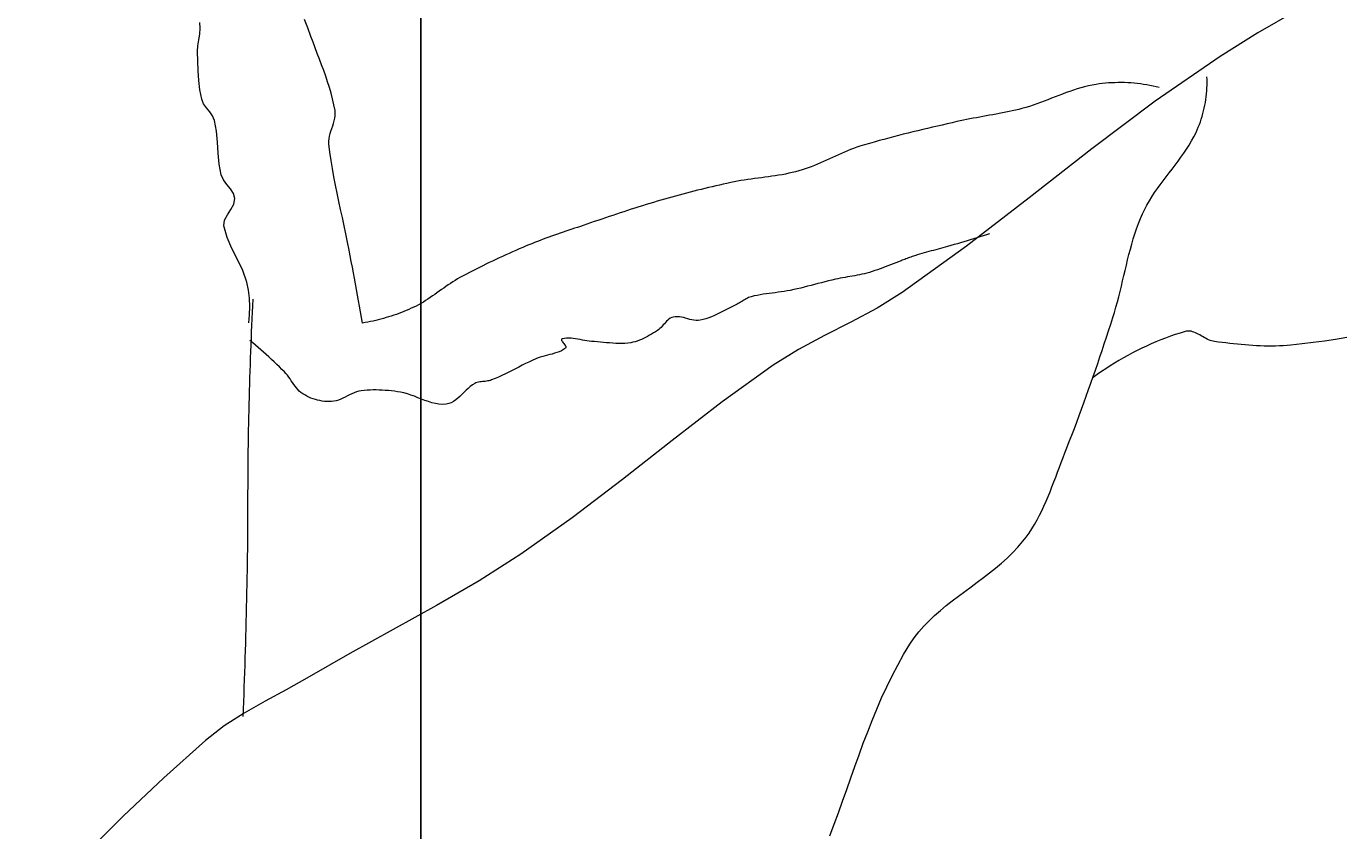
# Model space of a CAD drawing. Units: inches. Extents: x 1770 to 2988, y 1161 to 3221.
# Tile 15 of 44: x 2194 to 2229, y 2323 to 2344. Entities that reach past the tile are written whole.
import ezdxf

# ---------------------------------------------------------------- set-up
doc = ezdxf.new("R2010")
doc.units = ezdxf.units.IN
doc.layers.add('A-ANNO-DIMS', color=2, linetype='Continuous', lineweight=18)
doc.layers.add('A-FURN', color=8, linetype='Continuous', lineweight=13)
doc.styles.get("Standard").update_dxf_attribs({"font": 'arial.ttf'})
doc.dimstyles.get("Standard").update_dxf_attribs({"dimtxt": 0.18, "dimasz": 0.18, "dimexe": 0.18, "dimexo": 0.0625, "dimgap": 0.09, "dimtad": 0, "dimtih": 1, "dimtoh": 1, "dimdec": 4, "dimzin": 0, "dimdsep": 46, "dimtxsty": 'Standard', "dimcen": 0.09, "dimadec": 0, "dimazin": 0, "dimtfac": 1, "dimtdec": 4, "dimtofl": 0, "dimtmove": 0, "dimatfit": 3, "dimfxl": 1, "dimtolj": 1, "dimtzin": 0, "dimarcsym": 0})

# ---------------------------------------------------------------- blocks, each defined once
blk = doc.blocks.new('BED-DOUBLE-PLAN')
for p, q in [((8.372, 84.675), (8.284, 84.904)), ((34.877, 85.131), (33.846, 84.541)), ((5.475, 84.513), (5.49, 84.67)), ((5.49, 84.67), (5.478, 84.825)), ((8.458, 84.444), (8.372, 84.675)), ((33.846, 84.541), (32.841, 83.914)), ((5.415, 84.04), (5.424, 84.198)), ((5.424, 84.198), (5.448, 84.355)), ((5.448, 84.355), (5.475, 84.513)), ((8.513, 84.293), (8.458, 84.444)), ((8.57, 84.142), (8.513, 84.293)), ((5.421, 83.783), (5.415, 84.04)), ((8.628, 83.992), (8.57, 84.142)), ((8.685, 83.841), (8.628, 83.992)), ((8.743, 83.69), (8.685, 83.841)), ((32.841, 83.914), (31.092, 82.71)), ((5.43, 83.526), (5.421, 83.783)), ((5.447, 83.269), (5.43, 83.526)), ((8.799, 83.539), (8.743, 83.69)), ((8.853, 83.387), (8.799, 83.539)), ((5.478, 83.015), (5.447, 83.269)), ((8.905, 83.235), (8.853, 83.387)), ((8.954, 83.082), (8.905, 83.235)), ((29.405, 83.144), (29.303, 83.123)), ((29.508, 83.162), (29.405, 83.144)), ((29.592, 83.174), (29.508, 83.162)), ((29.676, 83.184), (29.592, 83.174)), ((29.761, 83.193), (29.676, 83.184)), ((29.846, 83.2), (29.761, 83.193)), ((29.931, 83.205), (29.846, 83.2)), ((30.016, 83.208), (29.931, 83.205)), ((30.102, 83.21), (30.016, 83.208)), ((30.187, 83.21), (30.102, 83.21)), ((30.273, 83.209), (30.187, 83.21)), ((30.358, 83.205), (30.273, 83.209)), ((30.444, 83.2), (30.358, 83.205)), ((30.529, 83.194), (30.444, 83.2)), ((30.614, 83.185), (30.529, 83.194)), ((30.699, 83.175), (30.614, 83.185)), ((30.784, 83.163), (30.699, 83.175)), ((30.868, 83.15), (30.784, 83.163)), ((30.952, 83.135), (30.868, 83.15)), ((31.036, 83.118), (30.952, 83.135)), ((32.486, 83.292), (32.483, 83.369)), ((32.483, 83.063), (32.486, 83.14)), ((32.487, 83.216), (32.486, 83.292)), ((32.486, 83.14), (32.487, 83.216)), ((5.528, 82.764), (5.478, 83.015)), ((8.999, 82.928), (8.954, 83.082)), ((9.039, 82.773), (8.999, 82.928)), ((9.075, 82.617), (9.039, 82.773)), ((28.314, 82.79), (28.216, 82.752)), ((28.411, 82.829), (28.314, 82.79)), ((28.509, 82.867), (28.411, 82.829)), ((28.607, 82.904), (28.509, 82.867)), ((28.705, 82.941), (28.607, 82.904)), ((28.804, 82.976), (28.705, 82.941)), ((28.902, 83.01), (28.804, 82.976)), ((29.002, 83.042), (28.902, 83.01)), ((29.102, 83.072), (29.002, 83.042)), ((29.202, 83.099), (29.102, 83.072)), ((29.303, 83.123), (29.202, 83.099)), ((31.119, 83.1), (31.036, 83.118)), ((31.201, 83.08), (31.119, 83.1)), ((32.453, 82.757), (32.463, 82.833)), ((32.463, 82.833), (32.472, 82.91)), ((32.472, 82.91), (32.478, 82.986)), ((32.478, 82.986), (32.483, 83.063)), ((5.579, 82.643), (5.528, 82.764)), ((5.656, 82.532), (5.579, 82.643)), ((5.743, 82.426), (5.656, 82.532)), ((5.82, 82.316), (5.743, 82.426)), ((9.104, 82.459), (9.075, 82.617)), ((9.111, 82.39), (9.104, 82.459)), ((27.176, 82.433), (27.089, 82.415)), ((27.263, 82.452), (27.176, 82.433)), ((27.35, 82.472), (27.263, 82.452)), ((27.436, 82.493), (27.35, 82.472)), ((27.522, 82.516), (27.436, 82.493)), ((27.623, 82.544), (27.522, 82.516)), ((27.723, 82.574), (27.623, 82.544)), ((27.822, 82.607), (27.723, 82.574)), ((27.921, 82.642), (27.822, 82.607)), ((28.02, 82.678), (27.921, 82.642)), ((28.118, 82.715), (28.02, 82.678)), ((28.216, 82.752), (28.118, 82.715)), ((31.092, 82.71), (29.393, 81.433)), ((32.374, 82.379), (32.393, 82.454)), ((32.393, 82.454), (32.411, 82.529)), ((32.411, 82.529), (32.427, 82.605)), ((32.427, 82.605), (32.441, 82.68)), ((32.441, 82.68), (32.453, 82.757)), ((5.872, 82.195), (5.82, 82.316)), ((5.926, 81.906), (5.872, 82.195)), ((9.041, 82.049), (9.064, 82.117)), ((9.064, 82.117), (9.083, 82.185)), ((9.083, 82.185), (9.099, 82.253)), ((9.099, 82.253), (9.108, 82.322)), ((9.108, 82.322), (9.111, 82.39)), ((25.385, 82.073), (25.254, 82.042)), ((25.516, 82.103), (25.385, 82.073)), ((25.647, 82.133), (25.516, 82.103)), ((25.778, 82.164), (25.647, 82.133)), ((25.865, 82.183), (25.778, 82.164)), ((25.952, 82.202), (25.865, 82.183)), ((26.039, 82.22), (25.952, 82.202)), ((26.126, 82.237), (26.039, 82.22)), ((26.214, 82.254), (26.126, 82.237)), ((26.301, 82.27), (26.214, 82.254)), ((26.389, 82.286), (26.301, 82.27)), ((26.477, 82.301), (26.389, 82.286)), ((26.564, 82.317), (26.477, 82.301)), ((26.652, 82.333), (26.564, 82.317)), ((26.74, 82.348), (26.652, 82.333)), ((26.827, 82.364), (26.74, 82.348)), ((26.915, 82.381), (26.827, 82.364)), ((27.002, 82.397), (26.915, 82.381)), ((27.089, 82.415), (27.002, 82.397)), ((32.251, 82.016), (32.279, 82.087)), ((32.279, 82.087), (32.305, 82.159)), ((32.305, 82.159), (32.33, 82.232)), ((32.33, 82.232), (32.353, 82.305)), ((32.353, 82.305), (32.374, 82.379)), ((5.953, 81.612), (5.926, 81.906)), ((8.944, 81.706), (8.956, 81.775)), ((8.956, 81.775), (8.974, 81.843)), ((8.974, 81.843), (8.995, 81.912)), ((8.995, 81.912), (9.018, 81.98)), ((9.018, 81.98), (9.041, 82.049)), ((23.949, 81.724), (23.819, 81.689)), ((24.079, 81.758), (23.949, 81.724)), ((24.209, 81.791), (24.079, 81.758)), ((24.339, 81.824), (24.209, 81.791)), ((24.47, 81.856), (24.339, 81.824)), ((24.6, 81.888), (24.47, 81.856)), ((24.731, 81.92), (24.6, 81.888)), ((24.862, 81.951), (24.731, 81.92)), ((24.992, 81.981), (24.862, 81.951)), ((25.123, 82.012), (24.992, 81.981)), ((25.254, 82.042), (25.123, 82.012)), ((32.069, 81.645), (32.132, 81.76)), ((32.132, 81.76), (32.189, 81.876)), ((32.189, 81.876), (32.221, 81.946)), ((32.221, 81.946), (32.251, 82.016)), ((5.971, 81.317), (5.953, 81.612)), ((8.938, 81.637), (8.944, 81.706)), ((8.94, 81.568), (8.938, 81.637)), ((8.966, 81.346), (8.94, 81.568)), ((22.843, 81.382), (22.762, 81.348)), ((22.925, 81.414), (22.843, 81.382)), ((23.008, 81.445), (22.925, 81.414)), ((23.091, 81.475), (23.008, 81.445)), ((23.174, 81.502), (23.091, 81.475)), ((23.303, 81.541), (23.174, 81.502)), ((23.431, 81.58), (23.303, 81.541)), ((23.56, 81.617), (23.431, 81.58)), ((23.69, 81.654), (23.56, 81.617)), ((23.819, 81.689), (23.69, 81.654)), ((29.393, 81.433), (27.716, 80.125)), ((31.86, 81.315), (31.933, 81.424)), ((31.933, 81.424), (32.003, 81.534)), ((32.003, 81.534), (32.069, 81.645)), ((5.998, 81.023), (5.971, 81.317)), ((6.052, 80.735), (5.998, 81.023)), ((8.996, 81.125), (8.966, 81.346)), ((9.032, 80.905), (8.996, 81.125)), ((22.037, 81.023), (21.955, 80.989)), ((22.118, 81.058), (22.037, 81.023)), ((22.198, 81.094), (22.118, 81.058)), ((22.279, 81.13), (22.198, 81.094)), ((22.359, 81.167), (22.279, 81.13)), ((22.439, 81.204), (22.359, 81.167)), ((22.52, 81.24), (22.439, 81.204)), ((22.6, 81.277), (22.52, 81.24)), ((22.681, 81.313), (22.6, 81.277)), ((22.762, 81.348), (22.681, 81.313)), ((31.628, 80.997), (31.707, 81.102)), ((31.707, 81.102), (31.784, 81.208)), ((31.784, 81.208), (31.86, 81.315)), ((6.113, 80.602), (6.052, 80.735)), ((9.071, 80.685), (9.032, 80.905)), ((9.114, 80.465), (9.071, 80.685)), ((20.537, 80.661), (20.445, 80.649)), ((20.63, 80.673), (20.537, 80.661)), ((20.722, 80.686), (20.63, 80.673)), ((20.814, 80.699), (20.722, 80.686)), ((20.905, 80.712), (20.814, 80.699)), ((20.997, 80.727), (20.905, 80.712)), ((21.088, 80.742), (20.997, 80.727)), ((21.18, 80.759), (21.088, 80.742)), ((21.27, 80.778), (21.18, 80.759)), ((21.361, 80.798), (21.27, 80.778)), ((21.451, 80.819), (21.361, 80.798)), ((21.54, 80.843), (21.451, 80.819)), ((21.625, 80.868), (21.54, 80.843)), ((21.708, 80.896), (21.625, 80.868)), ((21.791, 80.925), (21.708, 80.896)), ((21.873, 80.956), (21.791, 80.925)), ((21.955, 80.989), (21.873, 80.956)), ((31.309, 80.58), (31.388, 80.684)), ((31.388, 80.684), (31.468, 80.789)), ((31.468, 80.789), (31.548, 80.893)), ((31.548, 80.893), (31.628, 80.997)), ((6.204, 80.481), (6.113, 80.602)), ((6.301, 80.363), (6.204, 80.481)), ((6.381, 80.24), (6.301, 80.363)), ((9.159, 80.246), (9.114, 80.465)), ((18.724, 80.298), (18.625, 80.272)), ((18.822, 80.323), (18.724, 80.298)), ((18.921, 80.347), (18.822, 80.323)), ((19.019, 80.372), (18.921, 80.347)), ((19.118, 80.395), (19.019, 80.372)), ((19.217, 80.419), (19.118, 80.395)), ((19.316, 80.442), (19.217, 80.419)), ((19.415, 80.465), (19.316, 80.442)), ((19.514, 80.487), (19.415, 80.465)), ((19.613, 80.509), (19.514, 80.487)), ((19.712, 80.531), (19.613, 80.509)), ((19.803, 80.549), (19.712, 80.531)), ((19.894, 80.567), (19.803, 80.549)), ((19.985, 80.582), (19.894, 80.567)), ((20.077, 80.597), (19.985, 80.582)), ((20.169, 80.611), (20.077, 80.597)), ((20.261, 80.624), (20.169, 80.611)), ((20.353, 80.637), (20.261, 80.624)), ((20.445, 80.649), (20.353, 80.637)), ((31.079, 80.261), (31.154, 80.368)), ((31.154, 80.368), (31.231, 80.474)), ((31.231, 80.474), (31.309, 80.58)), ((6.311, 79.809), (6.39, 79.953)), ((6.418, 80.104), (6.381, 80.24)), ((6.39, 79.953), (6.418, 80.104)), ((9.205, 80.027), (9.159, 80.246)), ((9.253, 79.809), (9.205, 80.027)), ((17.544, 79.97), (17.444, 79.94)), ((17.644, 80), (17.544, 79.97)), ((17.744, 80.029), (17.644, 80)), ((17.842, 80.057), (17.744, 80.029)), ((17.939, 80.085), (17.842, 80.057)), ((18.037, 80.113), (17.939, 80.085)), ((18.135, 80.14), (18.037, 80.113)), ((18.233, 80.167), (18.135, 80.14)), ((18.331, 80.194), (18.233, 80.167)), ((18.429, 80.22), (18.331, 80.194)), ((18.527, 80.246), (18.429, 80.22)), ((18.625, 80.272), (18.527, 80.246)), ((27.716, 80.125), (26.032, 78.826)), ((30.874, 79.929), (30.939, 80.041)), ((30.939, 80.041), (31.008, 80.152)), ((31.008, 80.152), (31.079, 80.261)), ((6.144, 79.525), (6.217, 79.668)), ((6.217, 79.668), (6.311, 79.809)), ((9.302, 79.59), (9.253, 79.809)), ((9.349, 79.371), (9.302, 79.59)), ((16.451, 79.618), (16.352, 79.585)), ((16.55, 79.651), (16.451, 79.618)), ((16.649, 79.684), (16.55, 79.651)), ((16.748, 79.717), (16.649, 79.684)), ((16.847, 79.75), (16.748, 79.717)), ((16.946, 79.782), (16.847, 79.75)), ((17.046, 79.814), (16.946, 79.782)), ((17.145, 79.846), (17.046, 79.814)), ((17.245, 79.878), (17.145, 79.846)), ((17.344, 79.909), (17.245, 79.878)), ((17.444, 79.94), (17.344, 79.909)), ((30.7, 79.563), (30.757, 79.696)), ((30.757, 79.696), (30.813, 79.814)), ((30.813, 79.814), (30.874, 79.929)), ((6.126, 79.375), (6.144, 79.525)), ((6.207, 79.062), (6.126, 79.375)), ((9.396, 79.153), (9.349, 79.371)), ((15.373, 79.252), (15.296, 79.226)), ((15.45, 79.278), (15.373, 79.252)), ((15.527, 79.304), (15.45, 79.278)), ((15.605, 79.33), (15.527, 79.304)), ((15.682, 79.356), (15.605, 79.33)), ((15.759, 79.383), (15.682, 79.356)), ((15.858, 79.416), (15.759, 79.383)), ((15.957, 79.45), (15.858, 79.416)), ((16.055, 79.484), (15.957, 79.45)), ((16.154, 79.517), (16.055, 79.484)), ((16.253, 79.551), (16.154, 79.517)), ((16.352, 79.585), (16.253, 79.551)), ((30.551, 79.157), (30.597, 79.294)), ((30.597, 79.294), (30.647, 79.429)), ((30.647, 79.429), (30.7, 79.563)), ((6.338, 78.762), (6.207, 79.062)), ((9.441, 78.934), (9.396, 79.153)), ((9.484, 78.714), (9.441, 78.934)), ((14.376, 78.892), (14.301, 78.861)), ((14.452, 78.922), (14.376, 78.892)), ((14.528, 78.952), (14.452, 78.922)), ((14.604, 78.981), (14.528, 78.952)), ((14.68, 79.009), (14.604, 78.981)), ((14.757, 79.037), (14.68, 79.009)), ((14.833, 79.065), (14.757, 79.037)), ((14.91, 79.093), (14.833, 79.065)), ((14.987, 79.12), (14.91, 79.093)), ((15.064, 79.147), (14.987, 79.12)), ((15.141, 79.173), (15.064, 79.147)), ((15.218, 79.2), (15.141, 79.173)), ((15.296, 79.226), (15.218, 79.2)), ((25.79, 78.892), (25.703, 78.867)), ((25.876, 78.918), (25.79, 78.892)), ((25.963, 78.943), (25.876, 78.918)), ((26.05, 78.969), (25.963, 78.943)), ((26.136, 78.995), (26.05, 78.969)), ((26.223, 79.021), (26.136, 78.995)), ((26.31, 79.047), (26.223, 79.021)), ((26.396, 79.073), (26.31, 79.047)), ((26.483, 79.1), (26.396, 79.073)), ((26.569, 79.126), (26.483, 79.1)), ((26.656, 79.153), (26.569, 79.126)), ((30.467, 78.88), (30.508, 79.019)), ((30.508, 79.019), (30.551, 79.157)), ((6.489, 78.468), (6.338, 78.762)), ((9.512, 78.564), (9.484, 78.714)), ((9.54, 78.414), (9.512, 78.564)), ((13.595, 78.552), (13.506, 78.511)), ((13.685, 78.593), (13.595, 78.552)), ((13.775, 78.633), (13.685, 78.593)), ((13.865, 78.673), (13.775, 78.633)), ((13.955, 78.713), (13.865, 78.673)), ((14.045, 78.752), (13.955, 78.713)), ((14.135, 78.791), (14.045, 78.752)), ((14.225, 78.83), (14.135, 78.791)), ((14.301, 78.861), (14.225, 78.83)), ((26.032, 78.826), (24.311, 77.58)), ((24.544, 78.533), (24.511, 78.521)), ((24.577, 78.545), (24.544, 78.533)), ((24.61, 78.557), (24.577, 78.545)), ((24.643, 78.568), (24.61, 78.557)), ((24.676, 78.579), (24.643, 78.568)), ((24.71, 78.59), (24.676, 78.579)), ((24.772, 78.609), (24.71, 78.59)), ((24.835, 78.627), (24.772, 78.609)), ((24.898, 78.645), (24.835, 78.627)), ((24.961, 78.662), (24.898, 78.645)), ((25.024, 78.679), (24.961, 78.662)), ((25.087, 78.696), (25.024, 78.679)), ((25.151, 78.713), (25.087, 78.696)), ((25.214, 78.73), (25.151, 78.713)), ((25.277, 78.746), (25.214, 78.73)), ((25.34, 78.763), (25.277, 78.746)), ((25.403, 78.781), (25.34, 78.763)), ((25.466, 78.798), (25.403, 78.781)), ((25.529, 78.816), (25.466, 78.798)), ((25.616, 78.841), (25.529, 78.816)), ((25.703, 78.867), (25.616, 78.841)), ((30.356, 78.46), (30.391, 78.601)), ((30.391, 78.601), (30.428, 78.741)), ((30.428, 78.741), (30.467, 78.88)), ((6.633, 78.171), (6.489, 78.468)), ((9.568, 78.264), (9.54, 78.414)), ((9.596, 78.114), (9.568, 78.264)), ((12.887, 78.211), (12.799, 78.166)), ((12.974, 78.255), (12.887, 78.211)), ((13.063, 78.299), (12.974, 78.255)), ((13.151, 78.342), (13.063, 78.299)), ((13.239, 78.385), (13.151, 78.342)), ((13.328, 78.427), (13.239, 78.385)), ((13.417, 78.469), (13.328, 78.427)), ((13.506, 78.511), (13.417, 78.469)), ((23.646, 78.195), (23.575, 78.171)), ((23.717, 78.221), (23.646, 78.195)), ((23.788, 78.247), (23.717, 78.221)), ((23.858, 78.274), (23.788, 78.247)), ((23.928, 78.301), (23.858, 78.274)), ((23.999, 78.329), (23.928, 78.301)), ((24.069, 78.356), (23.999, 78.329)), ((24.139, 78.383), (24.069, 78.356)), ((24.21, 78.409), (24.139, 78.383)), ((24.28, 78.435), (24.21, 78.409)), ((24.313, 78.447), (24.28, 78.435)), ((24.346, 78.459), (24.313, 78.447)), ((24.379, 78.472), (24.346, 78.459)), ((24.412, 78.484), (24.379, 78.472)), ((24.445, 78.497), (24.412, 78.484)), ((24.478, 78.509), (24.445, 78.497)), ((24.511, 78.521), (24.478, 78.509)), ((30.254, 78.036), (30.288, 78.177)), ((30.288, 78.177), (30.321, 78.319)), ((30.321, 78.319), (30.356, 78.46)), ((6.741, 77.864), (6.633, 78.171)), ((6.786, 77.649), (6.741, 77.864)), ((9.623, 77.964), (9.596, 78.114)), ((9.651, 77.814), (9.623, 77.964)), ((12.2, 77.829), (12.139, 77.788)), ((12.262, 77.869), (12.2, 77.829)), ((12.324, 77.908), (12.262, 77.869)), ((12.387, 77.946), (12.324, 77.908)), ((12.452, 77.982), (12.387, 77.946)), ((12.538, 78.029), (12.452, 77.982)), ((12.625, 78.075), (12.538, 78.029)), ((12.712, 78.121), (12.625, 78.075)), ((12.799, 78.166), (12.712, 78.121)), ((22.053, 77.823), (21.961, 77.799)), ((22.146, 77.847), (22.053, 77.823)), ((22.239, 77.871), (22.146, 77.847)), ((22.332, 77.894), (22.239, 77.871)), ((22.425, 77.917), (22.332, 77.894)), ((22.518, 77.938), (22.425, 77.917)), ((22.583, 77.952), (22.518, 77.938)), ((22.648, 77.965), (22.583, 77.952)), ((22.713, 77.977), (22.648, 77.965)), ((22.778, 77.988), (22.713, 77.977)), ((22.843, 77.999), (22.778, 77.988)), ((22.908, 78.01), (22.843, 77.999)), ((22.973, 78.021), (22.908, 78.01)), ((23.038, 78.032), (22.973, 78.021)), ((23.103, 78.044), (23.038, 78.032)), ((23.168, 78.057), (23.103, 78.044)), ((23.232, 78.071), (23.168, 78.057)), ((23.296, 78.086), (23.232, 78.071)), ((23.36, 78.103), (23.296, 78.086)), ((23.432, 78.124), (23.36, 78.103)), ((23.504, 78.147), (23.432, 78.124)), ((23.575, 78.171), (23.504, 78.147)), ((30.188, 77.753), (30.221, 77.894)), ((30.221, 77.894), (30.254, 78.036)), ((6.813, 77.43), (6.786, 77.649)), ((9.678, 77.664), (9.651, 77.814)), ((9.706, 77.514), (9.678, 77.664)), ((9.733, 77.364), (9.706, 77.514)), ((11.717, 77.49), (11.656, 77.448)), ((11.777, 77.532), (11.717, 77.49)), ((11.837, 77.575), (11.777, 77.532)), ((11.897, 77.618), (11.837, 77.575)), ((11.957, 77.661), (11.897, 77.618)), ((12.018, 77.704), (11.957, 77.661)), ((12.078, 77.746), (12.018, 77.704)), ((12.139, 77.788), (12.078, 77.746)), ((20.261, 77.471), (20.227, 77.46)), ((20.34, 77.49), (20.261, 77.471)), ((20.42, 77.507), (20.34, 77.49)), ((20.5, 77.522), (20.42, 77.507)), ((20.581, 77.535), (20.5, 77.522)), ((20.662, 77.547), (20.581, 77.535)), ((20.743, 77.558), (20.662, 77.547)), ((20.824, 77.568), (20.743, 77.558)), ((20.905, 77.578), (20.824, 77.568)), ((20.986, 77.588), (20.905, 77.578)), ((21.067, 77.599), (20.986, 77.588)), ((21.148, 77.612), (21.067, 77.599)), ((21.229, 77.625), (21.148, 77.612)), ((21.309, 77.641), (21.229, 77.625)), ((21.402, 77.661), (21.309, 77.641)), ((21.496, 77.682), (21.402, 77.661)), ((21.589, 77.704), (21.496, 77.682)), ((21.682, 77.727), (21.589, 77.704)), ((21.775, 77.751), (21.682, 77.727)), ((21.868, 77.775), (21.775, 77.751)), ((21.961, 77.799), (21.868, 77.775)), ((24.311, 77.58), (23.639, 77.161)), ((30.081, 77.33), (30.118, 77.47)), ((30.118, 77.47), (30.153, 77.611)), ((30.153, 77.611), (30.188, 77.753)), ((6.823, 77.209), (6.813, 77.43)), ((6.814, 76.989), (6.823, 77.209)), ((6.89, 77.053), (6.898, 77.228)), ((6.898, 77.228), (6.907, 77.403)), ((9.76, 77.214), (9.733, 77.364)), ((9.787, 77.064), (9.76, 77.214)), ((11.082, 77.13), (11.015, 77.101)), ((11.147, 77.159), (11.082, 77.13)), ((11.213, 77.189), (11.147, 77.159)), ((11.279, 77.221), (11.213, 77.189)), ((11.344, 77.255), (11.279, 77.221)), ((11.408, 77.291), (11.344, 77.255)), ((11.471, 77.328), (11.408, 77.291)), ((11.533, 77.367), (11.471, 77.328)), ((11.595, 77.407), (11.533, 77.367)), ((11.656, 77.448), (11.595, 77.407)), ((19.636, 77.147), (19.564, 77.109)), ((19.709, 77.184), (19.636, 77.147)), ((19.781, 77.22), (19.709, 77.184)), ((19.854, 77.255), (19.781, 77.22)), ((19.886, 77.27), (19.854, 77.255)), ((19.917, 77.287), (19.886, 77.27)), ((19.948, 77.305), (19.917, 77.287)), ((19.978, 77.324), (19.948, 77.305)), ((20.008, 77.343), (19.978, 77.324)), ((20.039, 77.363), (20.008, 77.343)), ((20.069, 77.382), (20.039, 77.363)), ((20.1, 77.4), (20.069, 77.382)), ((20.131, 77.417), (20.1, 77.4)), ((20.162, 77.433), (20.131, 77.417)), ((20.194, 77.448), (20.162, 77.433)), ((20.227, 77.46), (20.194, 77.448)), ((23.639, 77.161), (22.938, 76.788)), ((30.002, 77.051), (30.043, 77.19)), ((30.043, 77.19), (30.081, 77.33)), ((6.788, 76.771), (6.814, 76.989)), ((6.875, 76.702), (6.883, 76.877)), ((6.883, 76.877), (6.89, 77.053)), ((9.814, 76.913), (9.787, 77.064)), ((9.841, 76.763), (9.814, 76.913)), ((9.912, 76.776), (9.841, 76.763)), ((9.982, 76.789), (9.912, 76.776)), ((10.053, 76.803), (9.982, 76.789)), ((10.123, 76.818), (10.053, 76.803)), ((10.194, 76.834), (10.123, 76.818)), ((10.264, 76.851), (10.194, 76.834)), ((10.333, 76.87), (10.264, 76.851)), ((10.403, 76.889), (10.333, 76.87)), ((10.472, 76.909), (10.403, 76.889)), ((10.541, 76.929), (10.472, 76.909)), ((10.61, 76.951), (10.541, 76.929)), ((10.678, 76.974), (10.61, 76.951)), ((10.747, 76.998), (10.678, 76.974)), ((10.814, 77.022), (10.747, 76.998)), ((10.882, 77.048), (10.814, 77.022)), ((10.949, 77.074), (10.882, 77.048)), ((11.015, 77.101), (10.949, 77.074)), ((17.965, 76.781), (17.935, 76.747)), ((17.995, 76.813), (17.965, 76.781)), ((18.026, 76.843), (17.995, 76.813)), ((18.058, 76.87), (18.026, 76.843)), ((18.093, 76.893), (18.058, 76.87)), ((18.13, 76.912), (18.093, 76.893)), ((18.17, 76.925), (18.13, 76.912)), ((18.225, 76.934), (18.17, 76.925)), ((18.28, 76.935), (18.225, 76.934)), ((18.336, 76.931), (18.28, 76.935)), ((18.391, 76.921), (18.336, 76.931)), ((18.447, 76.909), (18.391, 76.921)), ((18.503, 76.894), (18.447, 76.909)), ((18.56, 76.878), (18.503, 76.894)), ((18.616, 76.863), (18.56, 76.878)), ((18.672, 76.849), (18.616, 76.863)), ((18.728, 76.839), (18.672, 76.849)), ((18.784, 76.833), (18.728, 76.839)), ((18.839, 76.832), (18.784, 76.833)), ((18.894, 76.839), (18.839, 76.832)), ((18.973, 76.857), (18.894, 76.839)), ((19.049, 76.879), (18.973, 76.857)), ((19.125, 76.905), (19.049, 76.879)), ((19.2, 76.934), (19.125, 76.905)), ((19.274, 76.966), (19.2, 76.934)), ((19.347, 77), (19.274, 76.966)), ((19.42, 77.035), (19.347, 77)), ((19.492, 77.072), (19.42, 77.035)), ((19.564, 77.109), (19.492, 77.072)), ((22.938, 76.788), (22.227, 76.429)), ((29.902, 76.736), (29.959, 76.913)), ((29.959, 76.913), (30.002, 77.051)), ((6.861, 76.351), (6.868, 76.526)), ((6.868, 76.526), (6.875, 76.702)), ((17.483, 76.408), (17.429, 76.38)), ((17.536, 76.439), (17.483, 76.408)), ((17.589, 76.469), (17.536, 76.439)), ((17.642, 76.501), (17.589, 76.469)), ((17.694, 76.532), (17.642, 76.501)), ((17.746, 76.564), (17.694, 76.532)), ((17.781, 76.588), (17.746, 76.564)), ((17.815, 76.616), (17.781, 76.588)), ((17.846, 76.647), (17.815, 76.616)), ((17.877, 76.679), (17.846, 76.647)), ((17.906, 76.713), (17.877, 76.679)), ((17.935, 76.747), (17.906, 76.713)), ((22.227, 76.429), (21.526, 76.056)), ((29.786, 76.384), (29.844, 76.56)), ((29.844, 76.56), (29.902, 76.736)), ((31.503, 76.409), (31.372, 76.361)), ((31.633, 76.454), (31.503, 76.409)), ((31.765, 76.497), (31.633, 76.454)), ((31.897, 76.537), (31.765, 76.497)), ((31.936, 76.546), (31.897, 76.537)), ((31.976, 76.55), (31.936, 76.546)), ((32.016, 76.549), (31.976, 76.55)), ((32.055, 76.543), (32.016, 76.549)), ((32.094, 76.533), (32.055, 76.543)), ((32.133, 76.521), (32.094, 76.533)), ((32.172, 76.505), (32.133, 76.521)), ((32.211, 76.487), (32.172, 76.505)), ((32.249, 76.467), (32.211, 76.487)), ((32.288, 76.445), (32.249, 76.467)), ((32.327, 76.423), (32.288, 76.445)), ((32.366, 76.401), (32.327, 76.423)), ((6.895, 76.236), (6.82, 76.298)), ((6.847, 76), (6.854, 76.176)), ((6.854, 76.176), (6.861, 76.351)), ((6.969, 76.174), (6.895, 76.236)), ((7.042, 76.112), (6.969, 76.174)), ((7.115, 76.049), (7.042, 76.112)), ((15.229, 76.055), (15.172, 76.024)), ((15.18, 76.329), (15.176, 76.317)), ((15.176, 76.317), (15.18, 76.301)), ((15.194, 76.337), (15.18, 76.329)), ((15.18, 76.301), (15.19, 76.282)), ((15.19, 76.282), (15.205, 76.26)), ((15.253, 76.349), (15.194, 76.337)), ((15.205, 76.26), (15.223, 76.237)), ((15.223, 76.237), (15.242, 76.213)), ((15.282, 76.091), (15.229, 76.055)), ((15.242, 76.213), (15.26, 76.189)), ((15.312, 76.355), (15.253, 76.349)), ((15.26, 76.189), (15.276, 76.166)), ((15.276, 76.166), (15.288, 76.143)), ((15.293, 76.105), (15.282, 76.091)), ((15.288, 76.143), (15.295, 76.123)), ((15.295, 76.123), (15.293, 76.105)), ((15.372, 76.357), (15.312, 76.355)), ((15.432, 76.355), (15.372, 76.357)), ((15.492, 76.349), (15.432, 76.355)), ((15.553, 76.34), (15.492, 76.349)), ((15.614, 76.33), (15.553, 76.34)), ((15.675, 76.319), (15.614, 76.33)), ((15.736, 76.307), (15.675, 76.319)), ((15.797, 76.296), (15.736, 76.307)), ((15.858, 76.286), (15.797, 76.296)), ((15.918, 76.278), (15.858, 76.286)), ((15.979, 76.273), (15.918, 76.278)), ((16.06, 76.268), (15.979, 76.273)), ((16.141, 76.261), (16.06, 76.268)), ((16.222, 76.254), (16.141, 76.261)), ((16.304, 76.246), (16.222, 76.254)), ((16.385, 76.238), (16.304, 76.246)), ((16.466, 76.23), (16.385, 76.238)), ((16.548, 76.224), (16.466, 76.23)), ((16.629, 76.219), (16.548, 76.224)), ((16.71, 76.216), (16.629, 76.219)), ((16.791, 76.216), (16.71, 76.216)), ((16.871, 76.219), (16.791, 76.216)), ((16.952, 76.226), (16.871, 76.219)), ((17.032, 76.237), (16.952, 76.226)), ((17.091, 76.249), (17.032, 76.237)), ((17.149, 76.264), (17.091, 76.249)), ((17.207, 76.282), (17.149, 76.264)), ((17.263, 76.303), (17.207, 76.282)), ((17.319, 76.326), (17.263, 76.303)), ((17.374, 76.352), (17.319, 76.326)), ((17.429, 76.38), (17.374, 76.352)), ((21.526, 76.056), (20.852, 75.639)), ((29.67, 76.032), (29.728, 76.208)), ((29.728, 76.208), (29.786, 76.384)), ((30.734, 76.088), (30.61, 76.027)), ((30.86, 76.147), (30.734, 76.088)), ((30.987, 76.204), (30.86, 76.147)), ((31.115, 76.259), (30.987, 76.204)), ((31.243, 76.311), (31.115, 76.259)), ((31.372, 76.361), (31.243, 76.311)), ((32.406, 76.378), (32.366, 76.401)), ((32.445, 76.356), (32.406, 76.378)), ((32.485, 76.336), (32.445, 76.356)), ((32.524, 76.317), (32.485, 76.336)), ((32.564, 76.3), (32.524, 76.317)), ((32.605, 76.286), (32.564, 76.3)), ((32.646, 76.275), (32.605, 76.286)), ((32.687, 76.268), (32.646, 76.275)), ((32.789, 76.255), (32.687, 76.268)), ((32.89, 76.242), (32.789, 76.255)), ((32.992, 76.23), (32.89, 76.242)), ((33.094, 76.218), (32.992, 76.23)), ((33.196, 76.206), (33.094, 76.218)), ((33.299, 76.196), (33.196, 76.206)), ((33.401, 76.186), (33.299, 76.196)), ((33.503, 76.177), (33.401, 76.186)), ((33.606, 76.169), (33.503, 76.177)), ((33.708, 76.162), (33.606, 76.169)), ((33.811, 76.156), (33.708, 76.162)), ((33.913, 76.151), (33.811, 76.156)), ((34.016, 76.148), (33.913, 76.151)), ((34.118, 76.147), (34.016, 76.148)), ((34.221, 76.146), (34.118, 76.147)), ((34.323, 76.148), (34.221, 76.146)), ((34.425, 76.151), (34.323, 76.148)), ((34.527, 76.157), (34.425, 76.151)), ((34.629, 76.164), (34.527, 76.157)), ((34.731, 76.173), (34.629, 76.164)), ((35.032, 76.206), (34.731, 76.173)), ((35.332, 76.243), (35.032, 76.206)), ((35.632, 76.283), (35.332, 76.243)), ((35.931, 76.327), (35.632, 76.283)), ((36.23, 76.374), (35.931, 76.327)), ((6.835, 75.649), (6.841, 75.825)), ((6.841, 75.825), (6.847, 76)), ((7.188, 75.985), (7.115, 76.049)), ((7.26, 75.92), (7.188, 75.985)), ((7.331, 75.856), (7.26, 75.92)), ((7.402, 75.79), (7.331, 75.856)), ((7.472, 75.724), (7.402, 75.79)), ((7.542, 75.657), (7.472, 75.724)), ((14.301, 75.72), (14.21, 75.677)), ((14.393, 75.763), (14.301, 75.72)), ((14.485, 75.804), (14.393, 75.763)), ((14.546, 75.828), (14.485, 75.804)), ((14.608, 75.849), (14.546, 75.828)), ((14.671, 75.868), (14.608, 75.849)), ((14.735, 75.885), (14.671, 75.868)), ((14.8, 75.901), (14.735, 75.885)), ((14.864, 75.917), (14.8, 75.901)), ((14.928, 75.934), (14.864, 75.917)), ((14.991, 75.953), (14.928, 75.934)), ((15.053, 75.973), (14.991, 75.953)), ((15.114, 75.997), (15.053, 75.973)), ((15.172, 76.024), (15.114, 75.997)), ((29.552, 75.68), (29.611, 75.856)), ((29.611, 75.856), (29.67, 76.032)), ((30.122, 75.761), (30.003, 75.689)), ((30.242, 75.831), (30.122, 75.761)), ((30.363, 75.898), (30.242, 75.831)), ((30.486, 75.964), (30.363, 75.898)), ((30.61, 76.027), (30.486, 75.964)), ((6.823, 75.298), (6.829, 75.474)), ((6.829, 75.474), (6.835, 75.649)), ((7.611, 75.59), (7.542, 75.657)), ((7.68, 75.522), (7.611, 75.59)), ((7.748, 75.454), (7.68, 75.522)), ((7.788, 75.411), (7.748, 75.454)), ((7.826, 75.365), (7.788, 75.411)), ((7.861, 75.318), (7.826, 75.365)), ((13.579, 75.361), (13.487, 75.318)), ((13.67, 75.405), (13.579, 75.361)), ((13.76, 75.449), (13.67, 75.405)), ((13.85, 75.495), (13.76, 75.449)), ((13.94, 75.541), (13.85, 75.495)), ((14.03, 75.586), (13.94, 75.541)), ((14.12, 75.632), (14.03, 75.586)), ((14.21, 75.677), (14.12, 75.632)), ((20.852, 75.639), (19.481, 74.65)), ((29.542, 75.383), (29.431, 75.301)), ((29.432, 75.329), (29.492, 75.505)), ((29.492, 75.505), (29.552, 75.68)), ((29.655, 75.462), (29.542, 75.383)), ((29.77, 75.54), (29.655, 75.462)), ((29.886, 75.616), (29.77, 75.54)), ((30.003, 75.689), (29.886, 75.616)), ((6.812, 74.947), (6.818, 75.123)), ((6.818, 75.123), (6.823, 75.298)), ((7.896, 75.268), (7.861, 75.318)), ((7.929, 75.219), (7.896, 75.268)), ((7.962, 75.169), (7.929, 75.219)), ((7.996, 75.12), (7.962, 75.169)), ((8.031, 75.071), (7.996, 75.12)), ((8.067, 75.025), (8.031, 75.071)), ((8.105, 74.981), (8.067, 75.025)), ((12.671, 75.014), (12.615, 74.961)), ((12.728, 75.063), (12.671, 75.014)), ((12.788, 75.107), (12.728, 75.063)), ((12.851, 75.145), (12.788, 75.107)), ((12.883, 75.16), (12.851, 75.145)), ((12.916, 75.171), (12.883, 75.16)), ((12.95, 75.18), (12.916, 75.171)), ((12.985, 75.187), (12.95, 75.18)), ((13.02, 75.192), (12.985, 75.187)), ((13.056, 75.196), (13.02, 75.192)), ((13.092, 75.199), (13.056, 75.196)), ((13.128, 75.202), (13.092, 75.199)), ((13.164, 75.206), (13.128, 75.202)), ((13.199, 75.211), (13.164, 75.206)), ((13.234, 75.218), (13.199, 75.211)), ((13.269, 75.227), (13.234, 75.218)), ((13.302, 75.239), (13.269, 75.227)), ((13.395, 75.277), (13.302, 75.239)), ((13.487, 75.318), (13.395, 75.277)), ((29.31, 74.979), (29.371, 75.154)), ((29.371, 75.154), (29.432, 75.329)), ((6.803, 74.596), (6.807, 74.772)), ((6.807, 74.772), (6.812, 74.947)), ((8.146, 74.939), (8.105, 74.981)), ((8.189, 74.901), (8.146, 74.939)), ((8.237, 74.868), (8.189, 74.901)), ((8.29, 74.836), (8.237, 74.868)), ((8.344, 74.807), (8.29, 74.836)), ((8.4, 74.78), (8.344, 74.807)), ((8.458, 74.755), (8.4, 74.78)), ((8.516, 74.733), (8.458, 74.755)), ((8.576, 74.714), (8.516, 74.733)), ((8.636, 74.698), (8.576, 74.714)), ((8.697, 74.684), (8.636, 74.698)), ((8.759, 74.673), (8.697, 74.684)), ((8.82, 74.665), (8.759, 74.673)), ((8.882, 74.66), (8.82, 74.665)), ((8.944, 74.658), (8.882, 74.66)), ((9.005, 74.66), (8.944, 74.658)), ((9.07, 74.667), (9.005, 74.66)), ((9.133, 74.68), (9.07, 74.667)), ((9.194, 74.7), (9.133, 74.68)), ((9.255, 74.723), (9.194, 74.7)), ((9.315, 74.75), (9.255, 74.723)), ((9.375, 74.78), (9.315, 74.75)), ((9.435, 74.81), (9.375, 74.78)), ((9.494, 74.84), (9.435, 74.81)), ((9.554, 74.868), (9.494, 74.84)), ((9.615, 74.894), (9.554, 74.868)), ((9.676, 74.917), (9.615, 74.894)), ((9.739, 74.935), (9.676, 74.917)), ((9.803, 74.947), (9.739, 74.935)), ((9.883, 74.957), (9.803, 74.947)), ((9.964, 74.964), (9.883, 74.957)), ((10.045, 74.968), (9.964, 74.964)), ((10.126, 74.971), (10.045, 74.968)), ((10.207, 74.971), (10.126, 74.971)), ((10.289, 74.969), (10.207, 74.971)), ((10.37, 74.965), (10.289, 74.969)), ((10.452, 74.96), (10.37, 74.965)), ((10.533, 74.952), (10.452, 74.96)), ((10.614, 74.944), (10.533, 74.952)), ((10.695, 74.934), (10.614, 74.944)), ((10.775, 74.923), (10.695, 74.934)), ((10.856, 74.911), (10.775, 74.923)), ((10.951, 74.892), (10.856, 74.911)), ((11.046, 74.866), (10.951, 74.892)), ((11.14, 74.835), (11.046, 74.866)), ((11.234, 74.8), (11.14, 74.835)), ((11.327, 74.763), (11.234, 74.8)), ((11.421, 74.726), (11.327, 74.763)), ((11.514, 74.69), (11.421, 74.726)), ((11.607, 74.657), (11.514, 74.69)), ((11.7, 74.628), (11.607, 74.657)), ((12.279, 74.662), (12.217, 74.629)), ((12.338, 74.703), (12.279, 74.662)), ((12.396, 74.749), (12.338, 74.703)), ((12.451, 74.799), (12.396, 74.749)), ((12.506, 74.853), (12.451, 74.799)), ((12.56, 74.907), (12.506, 74.853)), ((12.615, 74.961), (12.56, 74.907)), ((19.481, 74.65), (18.14, 73.617)), ((29.185, 74.63), (29.248, 74.805)), ((29.248, 74.805), (29.31, 74.979)), ((6.794, 74.245), (6.798, 74.421)), ((6.798, 74.421), (6.803, 74.596)), ((11.794, 74.605), (11.7, 74.628)), ((11.889, 74.59), (11.794, 74.605)), ((11.984, 74.585), (11.889, 74.59)), ((12.08, 74.59), (11.984, 74.585)), ((12.151, 74.604), (12.08, 74.59)), ((12.217, 74.629), (12.151, 74.604)), ((29.058, 74.282), (29.122, 74.456)), ((29.122, 74.456), (29.185, 74.63)), ((6.786, 73.894), (6.79, 74.07)), ((6.79, 74.07), (6.794, 74.245)), ((28.86, 73.762), (28.927, 73.935)), ((28.927, 73.935), (28.993, 74.108)), ((28.993, 74.108), (29.058, 74.282)), ((6.779, 73.519), (6.782, 73.706)), ((6.782, 73.706), (6.786, 73.894)), ((18.14, 73.617), (16.81, 72.571)), ((28.724, 73.417), (28.792, 73.59)), ((28.792, 73.59), (28.86, 73.762)), ((6.775, 73.143), (6.777, 73.331)), ((6.777, 73.331), (6.779, 73.519)), ((28.623, 73.159), (28.673, 73.289)), ((28.673, 73.289), (28.724, 73.417)), ((6.772, 72.768), (6.773, 72.955)), ((6.773, 72.955), (6.775, 73.143)), ((28.476, 72.767), (28.525, 72.898)), ((28.525, 72.898), (28.574, 73.028)), ((28.574, 73.028), (28.623, 73.159)), ((6.77, 72.392), (6.771, 72.58)), ((6.771, 72.58), (6.772, 72.768)), ((16.81, 72.571), (15.466, 71.543)), ((28.377, 72.504), (28.427, 72.635)), ((28.427, 72.635), (28.476, 72.767)), ((6.769, 72.204), (6.77, 72.392)), ((6.769, 72.017), (6.769, 72.204)), ((28.222, 72.115), (28.275, 72.244)), ((28.275, 72.244), (28.327, 72.374)), ((28.327, 72.374), (28.377, 72.504)), ((6.767, 71.641), (6.768, 71.829)), ((6.768, 71.829), (6.769, 72.017)), ((28.052, 71.734), (28.111, 71.86)), ((28.111, 71.86), (28.168, 71.987)), ((28.168, 71.987), (28.222, 72.115)), ((6.766, 71.266), (6.767, 71.453)), ((6.767, 71.453), (6.767, 71.641)), ((15.466, 71.543), (14.086, 70.565)), ((27.858, 71.368), (27.926, 71.488)), ((27.926, 71.488), (27.99, 71.61)), ((27.99, 71.61), (28.052, 71.734)), ((6.765, 71.078), (6.766, 71.266)), ((27.631, 71.023), (27.711, 71.136)), ((27.711, 71.136), (27.786, 71.251)), ((27.786, 71.251), (27.858, 71.368)), ((6.762, 70.702), (6.763, 70.89)), ((6.763, 70.89), (6.765, 71.078)), ((27.275, 70.609), (27.415, 70.757)), ((27.415, 70.757), (27.547, 70.914)), ((27.547, 70.914), (27.631, 71.023)), ((6.757, 70.327), (6.759, 70.515)), ((6.759, 70.515), (6.762, 70.702)), ((14.086, 70.565), (12.968, 69.855)), ((26.975, 70.328), (27.128, 70.466)), ((27.128, 70.466), (27.275, 70.609)), ((6.75, 69.943), (6.754, 70.139)), ((6.754, 70.139), (6.757, 70.327)), ((26.491, 69.94), (26.655, 70.066)), ((26.655, 70.066), (26.817, 70.196)), ((26.817, 70.196), (26.975, 70.328)), ((6.742, 69.551), (6.746, 69.747)), ((6.746, 69.747), (6.75, 69.943)), ((12.968, 69.855), (11.823, 69.189)), ((25.988, 69.569), (26.156, 69.692)), ((26.156, 69.692), (26.324, 69.815)), ((26.324, 69.815), (26.491, 69.94)), ((6.733, 69.158), (6.737, 69.355)), ((6.737, 69.355), (6.742, 69.551)), ((25.655, 69.319), (25.82, 69.445)), ((25.82, 69.445), (25.988, 69.569)), ((6.728, 68.962), (6.733, 69.158)), ((11.823, 69.189), (10.663, 68.547)), ((25.181, 68.926), (25.335, 69.061)), ((25.335, 69.061), (25.493, 69.192)), ((25.493, 69.192), (25.655, 69.319)), ((6.718, 68.57), (6.723, 68.766)), ((6.723, 68.766), (6.728, 68.962)), ((24.759, 68.487), (24.892, 68.64)), ((24.892, 68.64), (25.033, 68.785)), ((25.033, 68.785), (25.181, 68.926)), ((6.708, 68.178), (6.713, 68.374)), ((6.713, 68.374), (6.718, 68.57)), ((10.663, 68.547), (9.501, 67.907)), ((24.52, 68.158), (24.635, 68.327)), ((24.635, 68.327), (24.759, 68.487)), ((6.696, 67.786), (6.702, 67.982)), ((6.702, 67.982), (6.708, 68.178)), ((24.35, 67.879), (24.52, 68.158)), ((6.684, 67.394), (6.69, 67.59)), ((6.69, 67.59), (6.696, 67.786)), ((9.501, 67.907), (8.35, 67.249)), ((24.039, 67.305), (24.19, 67.594)), ((24.19, 67.594), (24.35, 67.879)), ((6.678, 67.198), (6.684, 67.394)), ((8.35, 67.249), (7.792, 66.934)), ((23.895, 67.012), (24.039, 67.305)), ((6.664, 66.805), (6.671, 67.001)), ((6.671, 67.001), (6.678, 67.198)), ((7.792, 66.934), (7.227, 66.627)), ((23.759, 66.715), (23.895, 67.012)), ((6.65, 66.413), (6.657, 66.609)), ((6.657, 66.609), (6.664, 66.805)), ((7.227, 66.627), (6.669, 66.31)), ((23.629, 66.414), (23.759, 66.715)), ((6.669, 66.31), (6.131, 65.965)), ((6.643, 66.217), (6.65, 66.413)), ((23.505, 66.111), (23.629, 66.414)), ((6.131, 65.965), (5.627, 65.574)), ((23.268, 65.499), (23.385, 65.806)), ((23.385, 65.806), (23.505, 66.111)), ((5.627, 65.574), (4.51, 64.573)), ((23.155, 65.19), (23.268, 65.499)), ((23.043, 64.88), (23.155, 65.19)), ((22.933, 64.569), (23.043, 64.88)), ((4.51, 64.573), (3.42, 63.541)), ((22.823, 64.259), (22.933, 64.569)), ((22.712, 63.948), (22.823, 64.259)), ((22.6, 63.638), (22.712, 63.948)), ((3.42, 63.541), (2.36, 62.478)), ((22.367, 63.022), (22.485, 63.33)), ((22.485, 63.33), (22.6, 63.638))]:
    blk.add_line(p, q)
blk = doc.blocks.new('*D73')
at = {"layer": 'A-ANNO-DIMS', "color": 0, "lineweight": -2, "transparency": 16777216}
for p, q in [((2456.133, 2367.702), (1907.104, 2367.702)), ((1907.284, 2367.522), (1907.284, 2319.884)), ((1907.284, 2271.882), (1907.284, 2319.52)), ((2456.133, 2271.702), (1907.104, 2271.702))]:
    blk.add_line(p, q, dxfattribs=at)
at = {"layer": 'A-ANNO-DIMS', "color": 0, "transparency": 16777216}
for points in [[(1907.254, 2367.522), (1907.314, 2367.522), (1907.284, 2367.702)], [(1907.254, 2271.882), (1907.314, 2271.882), (1907.284, 2271.702)]]:
    blk.add_solid(points, dxfattribs=at)
at = {"layer": 'Defpoints', "color": 0, "transparency": 16777216}
for p in [(1907.284, 2367.702), (2456.196, 2367.702), (2456.196, 2271.702)]:
    blk.add_point(p, dxfattribs=at)
at = {"layer": 'A-ANNO-DIMS', "color": 0, "transparency": 16777216, "insert": (1907.284, 2319.702), "char_height": 0.18, "attachment_point": 5}
blk.add_mtext('\\A1;96', dxfattribs=at)
blk = doc.blocks.new('*D79')
at = {"layer": 'A-ANNO-DIMS', "color": 0, "lineweight": -2, "transparency": 16777216}
for p, q in [((2151.696, 1610.265), (2151.696, 2570.705)), ((2204.657, 1610.265), (2204.657, 2570.705)), ((2151.876, 2570.525), (2177.783, 2570.525)), ((2204.477, 2570.525), (2178.57, 2570.525))]:
    blk.add_line(p, q, dxfattribs=at)
at = {"layer": 'A-ANNO-DIMS', "color": 0, "transparency": 16777216}
for points in [[(2151.876, 2570.555), (2151.876, 2570.495), (2151.696, 2570.525)], [(2204.477, 2570.555), (2204.477, 2570.495), (2204.657, 2570.525)]]:
    blk.add_solid(points, dxfattribs=at)
at = {"layer": 'Defpoints', "color": 0, "transparency": 16777216}
for p in [(2204.657, 2570.525), (2151.696, 1610.202), (2204.657, 1610.202)]:
    blk.add_point(p, dxfattribs=at)
at = {"layer": 'A-ANNO-DIMS', "color": 0, "transparency": 16777216, "insert": (2178.176, 2570.525), "char_height": 0.18, "attachment_point": 5}
blk.add_mtext('\\A1;52.96', dxfattribs=at)

msp = doc.modelspace()

# ---------------------------------------------------------------- block references
at = {"layer": 'A-FURN'}
msp.add_blockref('BED-DOUBLE-PLAN', (2193.254, 2259.498), dxfattribs=at)

# ---------------------------------------------------------------- dimensions: what is measured, and where the dimension line sits
at = {"layer": 'A-ANNO-DIMS'}
dim = msp.add_linear_dim(base=(2204.6568, 2570.5247), p1=(2151.696, 1610.2021), p2=(2204.6568, 1610.2021), dimstyle='Standard', override={"dimdec": 2, "dimlfac": 1, "dimrnd": 0, "dimzin": 0, "dimdsep": 46, "dimlunit": 2}, dxfattribs=at)
dim.commit()
dim.dimension.update_dxf_attribs({"geometry": '*D79', "text_midpoint": (2178.1764, 2570.5247)})
dim = msp.add_linear_dim(base=(1907.2844, 2367.7021), p1=(2456.196, 2271.7021), p2=(2456.196, 2367.7021), angle=90, dimstyle='Standard', override={"dimdec": 0, "dimlfac": 1, "dimrnd": 0, "dimzin": 0, "dimdsep": 46, "dimlunit": 2}, dxfattribs=at)
dim.commit()
dim.dimension.update_dxf_attribs({"geometry": '*D73', "text_midpoint": (1907.2844, 2319.7021)})

doc.saveas('drawing.dxf')
